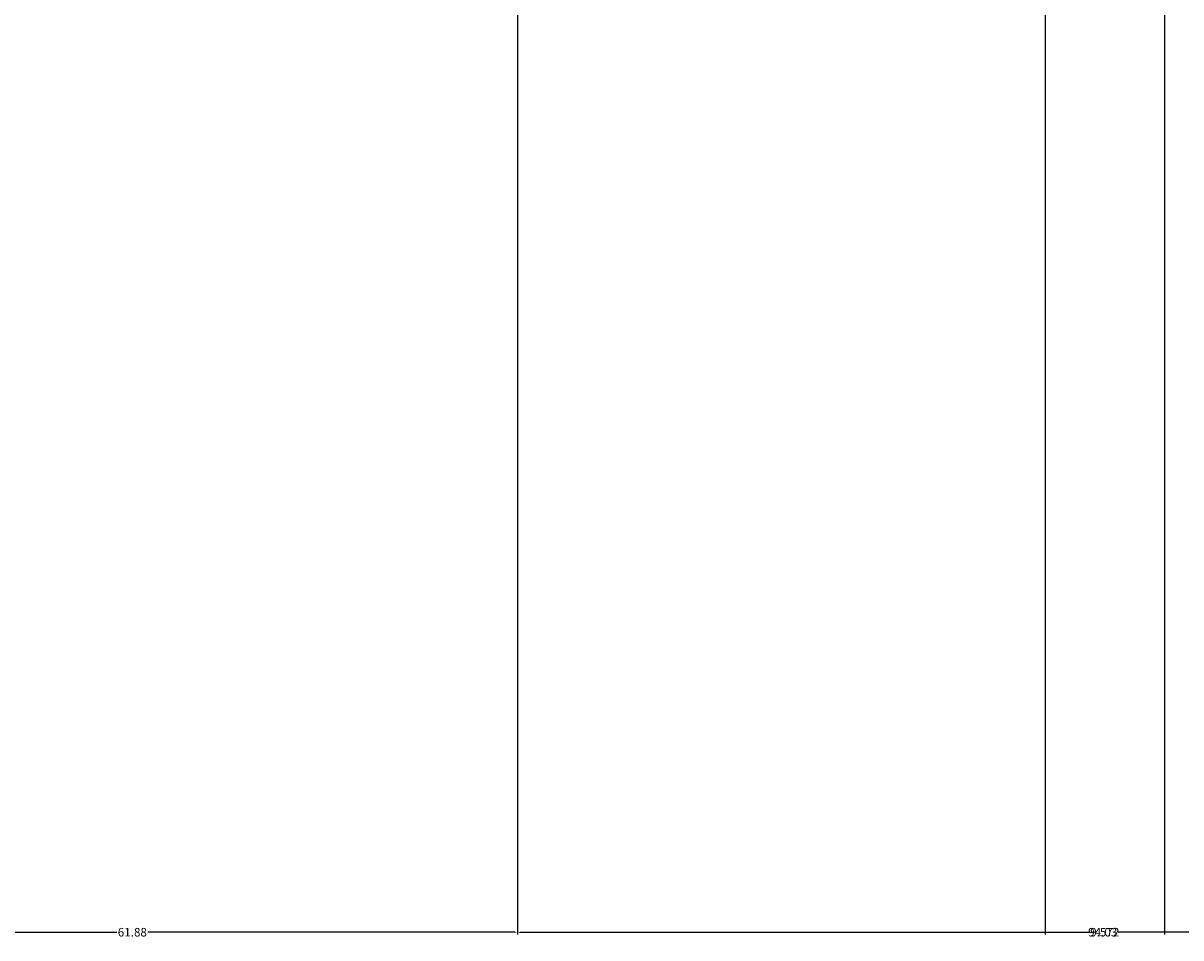
# Model space of a CAD drawing. Units: inches. Extents: x -145 to 510, y 5 to 386.
# Tile 14 of 25: x 182 to 275, y 5 to 78. Entities that reach past the tile are written whole.
import ezdxf

# ---------------------------------------------------------------- set-up
doc = ezdxf.new("R2010")
doc.units = ezdxf.units.IN
doc.header["$MEASUREMENT"] = 0
doc.layers.add('A-ANNO-DIMS', color=2, linetype='Continuous', lineweight=18)
doc.styles.get("Standard").update_dxf_attribs({"font": 'arial.ttf'})
doc.dimstyles.get("Standard").update_dxf_attribs({"dimtxt": 0.6875, "dimasz": 0.18, "dimexe": 0.18, "dimexo": 0.0625, "dimgap": 0.09, "dimtad": 0, "dimtih": 1, "dimtoh": 1, "dimdec": 4, "dimzin": 0, "dimdsep": 46, "dimlunit": 4, "dimtxsty": 'Standard', "dimcen": 0.09, "dimadec": 0, "dimazin": 0, "dimtfac": 1, "dimtdec": 4, "dimtofl": 0, "dimtmove": 0, "dimatfit": 3, "dimfxl": 1, "dimtolj": 1, "dimtzin": 0, "dimarcsym": 0})

# ---------------------------------------------------------------- blocks, each defined once
blk = doc.blocks.new('*D9')
at = {"layer": 'A-ANNO-DIMS', "color": 0, "lineweight": -2, "transparency": 16777216}
for p, q in [((159.649, 115.23), (159.649, 5.194)), ((221.529, 85.201), (221.529, 5.194)), ((159.829, 5.374), (189.337, 5.374)), ((221.349, 5.374), (191.842, 5.374))]:
    blk.add_line(p, q, dxfattribs=at)
at = {"layer": 'A-ANNO-DIMS', "color": 0, "transparency": 16777216}
for points in [[(159.829, 5.404), (159.829, 5.344), (159.649, 5.374)], [(221.349, 5.404), (221.349, 5.344), (221.529, 5.374)]]:
    blk.add_solid(points, dxfattribs=at)
at = {"layer": 'Defpoints', "color": 0, "transparency": 16777216}
for p in [(159.649, 115.292), (221.529, 85.264), (221.529, 5.374)]:
    blk.add_point(p, dxfattribs=at)
at = {"layer": 'A-ANNO-DIMS', "color": 0, "transparency": 16777216, "insert": (190.589, 5.374), "char_height": 0.6875, "attachment_point": 5}
blk.add_mtext('\\A1;61.88', dxfattribs=at)
blk = doc.blocks.new('*D10')
at = {"layer": 'A-ANNO-DIMS', "color": 0, "lineweight": -2, "transparency": 16777216}
for p, q in [((221.529, 85.201), (221.529, 5.194)), ((315.554, 85.201), (315.554, 5.194)), ((221.709, 5.374), (267.292, 5.374)), ((315.374, 5.374), (269.792, 5.374))]:
    blk.add_line(p, q, dxfattribs=at)
at = {"layer": 'A-ANNO-DIMS', "color": 0, "transparency": 16777216}
for points in [[(221.709, 5.404), (221.709, 5.344), (221.529, 5.374)], [(315.374, 5.404), (315.374, 5.344), (315.554, 5.374)]]:
    blk.add_solid(points, dxfattribs=at)
at = {"layer": 'Defpoints', "color": 0, "transparency": 16777216}
for p in [(221.529, 85.264), (315.554, 85.264), (315.554, 5.374)]:
    blk.add_point(p, dxfattribs=at)
at = {"layer": 'A-ANNO-DIMS', "color": 0, "transparency": 16777216, "insert": (268.542, 5.374), "char_height": 0.6875, "attachment_point": 5}
blk.add_mtext('\\A1;94.03', dxfattribs=at)
blk = doc.blocks.new('*D56')
at = {"layer": 'A-ANNO-DIMS', "color": 0, "lineweight": -2, "transparency": 16777216}
for p, q in [((273.491, 156.547), (273.491, 5.194)), ((263.918, 130.608), (263.918, 5.194)), ((264.098, 5.374), (267.458, 5.374)), ((273.311, 5.374), (269.951, 5.374))]:
    blk.add_line(p, q, dxfattribs=at)
at = {"layer": 'A-ANNO-DIMS', "color": 0, "transparency": 16777216}
for points in [[(264.098, 5.404), (264.098, 5.344), (263.918, 5.374)], [(273.311, 5.404), (273.311, 5.344), (273.491, 5.374)]]:
    blk.add_solid(points, dxfattribs=at)
at = {"layer": 'Defpoints', "color": 0, "transparency": 16777216}
for p in [(273.491, 156.609), (263.918, 130.671), (273.491, 5.374)]:
    blk.add_point(p, dxfattribs=at)
at = {"layer": 'A-ANNO-DIMS', "color": 0, "transparency": 16777216, "insert": (268.704, 5.374), "char_height": 0.6875, "attachment_point": 5}
blk.add_mtext('\\A1;9.572', dxfattribs=at)

msp = doc.modelspace()

# ---------------------------------------------------------------- dimensions: what is measured, and where the dimension line sits
at = {"layer": 'A-ANNO-DIMS'}
for base, p1, p2, override, picture, middle in [((273.4905, 5.3738), (263.9183, 130.6707), (273.4905, 156.6093), {"dimdec": 3, "dimlfac": 1, "dimrnd": 0, "dimzin": 0, "dimdsep": 46, "dimlunit": 2}, '*D56', (268.7044, 5.3738)), ((221.5292, 5.3738), (159.6492, 115.2922), (221.5292, 85.2638), {"dimdec": 2, "dimlfac": 1, "dimrnd": 0, "dimzin": 0, "dimdsep": 46, "dimlunit": 2}, '*D9', (190.5892, 5.3738)), ((315.5545, 5.3738), (221.5292, 85.2638), (315.5545, 85.2638), {"dimdec": 2, "dimlfac": 1, "dimrnd": 0, "dimzin": 0, "dimdsep": 46, "dimlunit": 2}, '*D10', (268.5418, 5.3738))]:
    dim = msp.add_linear_dim(base=base, p1=p1, p2=p2, dimstyle='Standard', override=override, dxfattribs=at)
    dim.commit()
    dim.dimension.update_dxf_attribs({"geometry": picture, "text_midpoint": middle})

doc.saveas('drawing.dxf')
